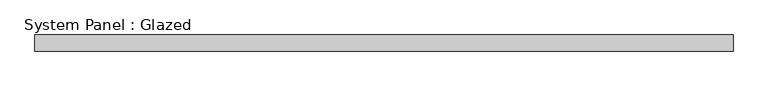
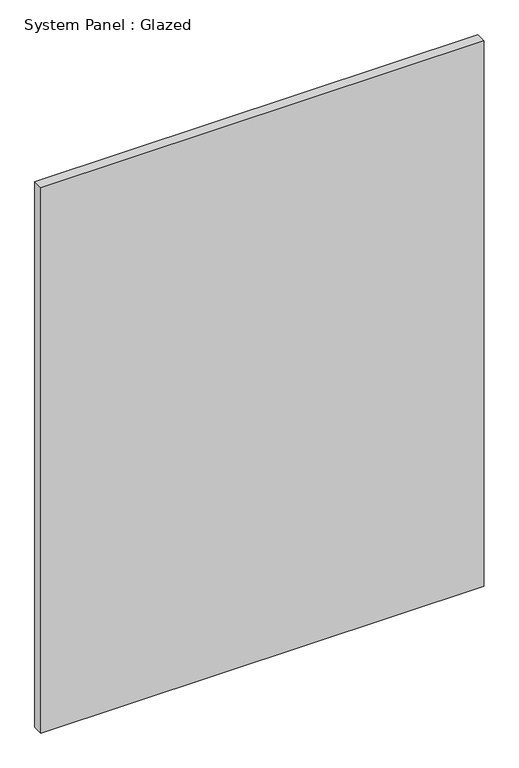
"""IFC4 building model written with IfcOpenShell, lengths in millimetres: plate geometry, System Panel : Glazed."""

from ifc_helpers import new_model, si_unit, origin, origin_with_axes, place, context, project, spatial, polyline, outline, extrude, source, transform, mapped, element, save


def system_panel_glazed_cbd410f7(model_context):
    return source(origin(), model_context, "Body", "SweptSolid", [
        extrude(outline(polyline([(536.575, 19.05), (-536.575, 19.05), (-536.575, 44.45), (536.575, 44.45), (536.575, 19.05)])), origin_with_axes(), (0.0, 0.0, 1.0), 1396.1033231),
    ])


if __name__ == "__main__":
    model = new_model("IFC4")
    model_context = context("Model", 3, world=origin())
    ifc_project = project(units=[si_unit("LENGTHUNIT", "METRE", prefix="MILLI")], contexts=[model_context])
    site = spatial("IfcSite", under=ifc_project)
    building = spatial("IfcBuilding", under=site)
    placement = place(None, origin())
    system_panel_glazed_shape = system_panel_glazed_cbd410f7(model_context)
    element("IfcPlate", 1, ObjectType="System Panel : Glazed", at=placement, inside=building, context=model_context, shape_type="MappedRepresentation", body=[
        mapped(system_panel_glazed_shape, transform((0.0, 0.0, 0.0), x_axis=(1.0, 0.0, 0.0), y_axis=(0.0, 1.0, 0.0), z_axis=(0.0, 0.0, 1.0))),
    ])
    save(model, "model.ifc")

# Revit data of these elements
# Type "System Panel : Glazed"
#   Construction Type Id = "GSP4R"
#   Analytic Construction = "1/8 in Pilkington single glazing"
#   Visual Light Transmittance = 0.9
#   Solar Heat Gain Coefficient = 0.86
#   Heat Transfer Coefficient (U) = 1.18115 BTU/(h·ft²·°F)
#   Define Thermal Properties by = 1
# Element 1 (IfcPlate, "System Panel : Glazed")
#   Materials on its faces: "Glass"
# Materials
#   "Glass": class "Glass", colour RGB 0 128 192, transparency 0.75, Description = "Soda Lime Glass", Cost = 0
